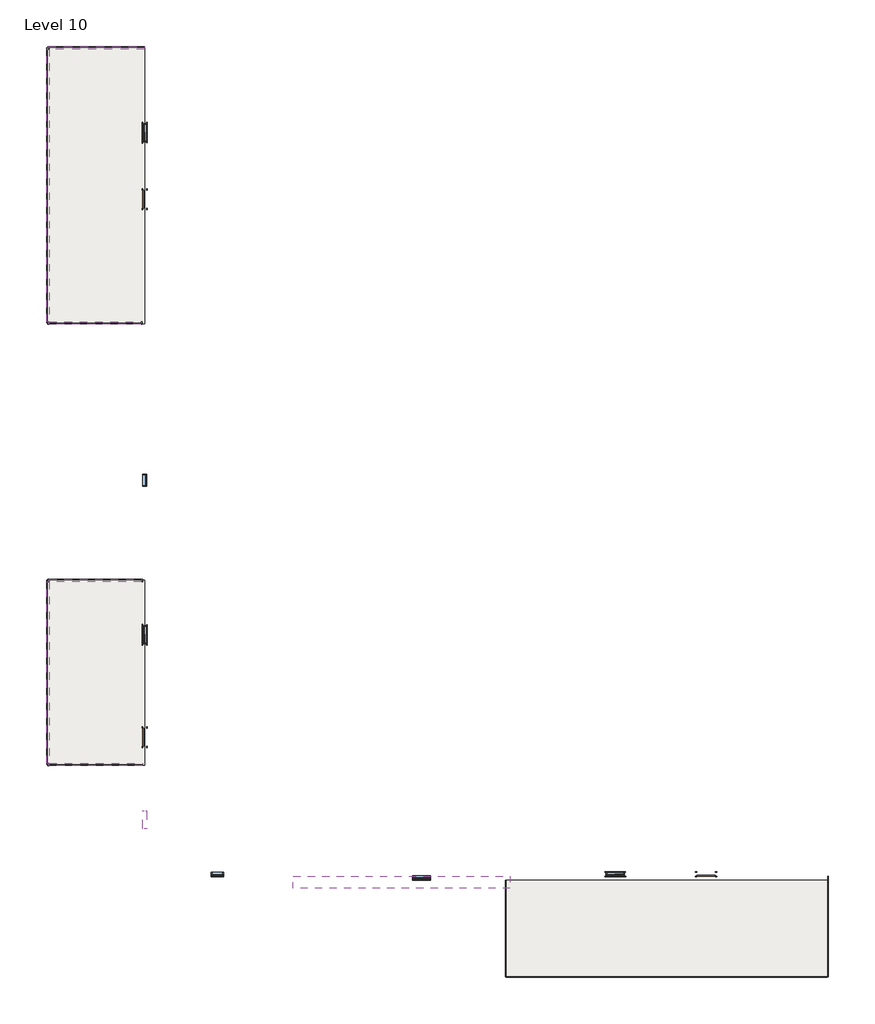
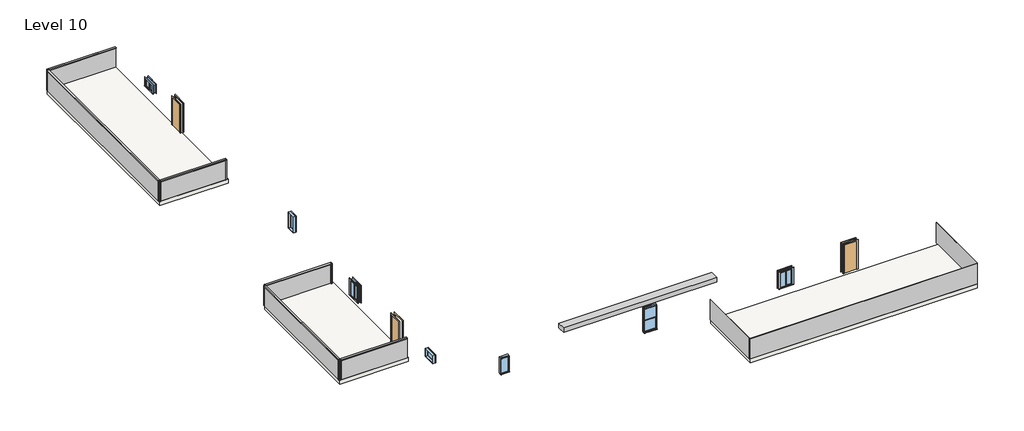
# One storey: 15 members, 9 plates, 7 windows, 3 doors, 3 slabs, 1 proxy.
"""IFC4 building model written with IfcOpenShell, lengths in millimetres."""

from ifc_helpers import new_model, si_unit, frame, origin, place, context, project, spatial, polyline, outline, extrude, transform, mapped, element, save
from components import generic_models_6_generic_models_6_4e89bfb7, door_54dd4da4, door_719f80de, member_4491d118, member_6d14b308, member_5c8c9790, member_b978f1c8, member_fc9bce7c, member_e4af79e9, member_f5ad0230, system_panel_glazed_dbf8c7ac, system_panel_glazed_4eae45b3, system_panel_glazed_9244b5db, system_panel_glazed_1f759628, system_panel_glazed_f6bd2989, system_panel_glazed_6e908680, system_panel_glazed_242742f8, system_panel_glazed_7dd8e57f, system_panel_glazed_8414a7a5, window_f274a882, window_80bd9af0, window_57c3ee1c, window_78885257, window_a4355bb3, window_54100e87

model = new_model("IFC4")

# Units and contexts
model_context = context("Model", 3, world=origin())
ifc_project = project(units=[si_unit("LENGTHUNIT", "METRE", prefix="MILLI")], contexts=[model_context])

# Site, building, storey
site = spatial("IfcSite", under=ifc_project)
building = spatial("IfcBuilding", under=site)
storey = spatial("IfcBuildingStorey", under=building, Name="Level 10", Elevation=16459.2)

# Proxy
placement = place(None, origin())
generic_models_6_generic_models_6_shape = generic_models_6_generic_models_6_4e89bfb7(model_context)
element("IfcBuildingElementProxy", 1, Name="Generic Models 6 : Generic Models 6", ObjectType="Generic Models 6 : Generic Models 6", at=placement, inside=storey, context=model_context, shape_type="MappedRepresentation", body=[
    mapped(generic_models_6_generic_models_6_shape, transform((0.0, 0.0, 0.0), x_axis=(1.0, 0.0, 0.0), y_axis=(0.0, 1.0, 0.0), z_axis=(0.0, 0.0, 1.0))),
])

# Doors
door_shape = door_54dd4da4(model_context)
element("IfcDoor", 2, ObjectType="Single-Flush : 36\" x 84\"", at=placement, inside=storey, context=model_context, shape_type="MappedRepresentation", body=[
    mapped(door_shape, transform((-15175.038074, 13190.2014639, 16459.2), x_axis=(0.0, 1.0, 0.0), y_axis=(-1.0, 0.0, 0.0), z_axis=(0.0, 0.0, 1.0))),
])
element("IfcDoor", 3, ObjectType="Single-Flush : 36\" x 84\"", at=placement, inside=storey, context=model_context, shape_type="MappedRepresentation", body=[
    mapped(door_shape, transform((-15175.038074, -13852.5915889, 16459.2), x_axis=(0.0, 1.0, 0.0), y_axis=(-1.0, 0.0, 0.0), z_axis=(0.0, 0.0, 1.0))),
])
door_2_shape = door_719f80de(model_context)
element("IfcDoor", 4, ObjectType="Single-Flush : 36\" x 84\"", at=placement, inside=storey, context=model_context, shape_type="MappedRepresentation", body=[
    mapped(door_2_shape, transform((13069.761926, -20744.1985361, 16459.2), x_axis=(1.0, 0.0, 0.0), y_axis=(0.0, 1.0, 0.0), z_axis=(0.0, 0.0, 1.0))),
])

# Members
member_shape = member_4491d118(model_context)
element("IfcMember", 5, ObjectType="Rectangular Mullion : 2.5\" x 5\" rectangular", at=placement, inside=storey, context=model_context, shape_type="MappedRepresentation", body=[
    mapped(member_shape, transform((-20051.838074, 6979.9014639, 16459.2), x_axis=(-1.0, 0.0, 0.0), y_axis=(0.0, 1.0, 0.0), z_axis=(0.0, 0.0, -1.0))),
])
element("IfcMember", 6, ObjectType="Rectangular Mullion : 2.5\" x 5\" rectangular", at=placement, inside=storey, context=model_context, shape_type="MappedRepresentation", body=[
    mapped(member_shape, transform((-20051.838074, 20810.2014639, 16459.2), x_axis=(0.0, 1.0, 0.0), y_axis=(1.0, 0.0, 0.0), z_axis=(0.0, 0.0, -1.0))),
])
element("IfcMember", 7, ObjectType="Rectangular Mullion : 2.5\" x 5\" rectangular", at=placement, inside=storey, context=model_context, shape_type="MappedRepresentation", body=[
    mapped(member_shape, transform((-20051.838074, -15224.1915889, 16459.2), x_axis=(-1.0, 0.0, 0.0), y_axis=(0.0, 1.0, 0.0), z_axis=(0.0, 0.0, -1.0))),
])
element("IfcMember", 8, ObjectType="Rectangular Mullion : 2.5\" x 5\" rectangular", at=placement, inside=storey, context=model_context, shape_type="MappedRepresentation", body=[
    mapped(member_shape, transform((-15276.638074, -5966.8213044, 16459.2), x_axis=(1.0, 0.0, 0.0), y_axis=(0.0, -1.0, 0.0), z_axis=(0.0, 0.0, -1.0))),
])
element("IfcMember", 9, ObjectType="Rectangular Mullion : 2.5\" x 5\" rectangular", at=placement, inside=storey, context=model_context, shape_type="MappedRepresentation", body=[
    mapped(member_shape, transform((-20051.838074, -5966.8213044, 16459.2), x_axis=(0.0, 1.0, 0.0), y_axis=(1.0, 0.0, 0.0), z_axis=(0.0, 0.0, -1.0))),
])
element("IfcMember", 10, ObjectType="Rectangular Mullion : 2.5\" x 5\" rectangular", at=placement, inside=storey, context=model_context, shape_type="MappedRepresentation", body=[
    mapped(member_shape, transform((-20051.838074, 6979.9014639, 17983.2), x_axis=(0.0, -1.0, 0.0), y_axis=(1.0, 0.0, 0.0), z_axis=(0.0, 0.0, 1.0))),
])
element("IfcMember", 11, ObjectType="Rectangular Mullion : 2.5\" x 5\" rectangular", at=placement, inside=storey, context=model_context, shape_type="MappedRepresentation", body=[
    mapped(member_shape, transform((-15295.688074, 6979.9014639, 17983.2), x_axis=(1.0, 0.0, 0.0), y_axis=(0.0, 1.0, 0.0), z_axis=(0.0, 0.0, 1.0))),
])
element("IfcMember", 12, ObjectType="Rectangular Mullion : 2.5\" x 5\" rectangular", at=placement, inside=storey, context=model_context, shape_type="MappedRepresentation", body=[
    mapped(member_shape, transform((-20051.838074, -15224.1915889, 17983.2), x_axis=(0.0, -1.0, 0.0), y_axis=(1.0, 0.0, 0.0), z_axis=(0.0, 0.0, 1.0))),
])
element("IfcMember", 13, ObjectType="Rectangular Mullion : 2.5\" x 5\" rectangular", at=placement, inside=storey, context=model_context, shape_type="MappedRepresentation", body=[
    mapped(member_shape, transform((-20051.838074, -5966.8213044, 17983.2), x_axis=(-1.0, 0.0, 0.0), y_axis=(0.0, -1.0, 0.0), z_axis=(0.0, 0.0, 1.0))),
])
member_2_shape = member_6d14b308(model_context)
element("IfcMember", 14, ObjectType="Rectangular Mullion : 2.5\" x 5\" rectangular", at=placement, inside=storey, context=model_context, shape_type="MappedRepresentation", body=[
    mapped(member_2_shape, transform((-15340.138074, -5966.8213044, 17983.2), x_axis=(0.0, 0.0, 1.0), y_axis=(0.0, -1.0, 0.0), z_axis=(1.0, 0.0, 0.0))),
])
member_3_shape = member_5c8c9790(model_context)
element("IfcMember", 15, ObjectType="Rectangular Mullion : 2.5\" x 5\" rectangular", at=placement, inside=storey, context=model_context, shape_type="MappedRepresentation", body=[
    mapped(member_3_shape, transform((-19988.338074, 6979.9014639, 17983.2), x_axis=(0.0, 0.0, 1.0), y_axis=(0.0, 1.0, 0.0), z_axis=(-1.0, 0.0, 0.0))),
])
member_4_shape = member_b978f1c8(model_context)
element("IfcMember", 16, ObjectType="Rectangular Mullion : 2.5\" x 5\" rectangular", at=placement, inside=storey, context=model_context, shape_type="MappedRepresentation", body=[
    mapped(member_4_shape, transform((-20051.838074, 20746.7014639, 17983.2), x_axis=(0.0, 0.0, 1.0), y_axis=(1.0, 0.0, 0.0), z_axis=(0.0, 1.0, 0.0))),
])
member_5_shape = member_fc9bce7c(model_context)
element("IfcMember", 17, ObjectType="Rectangular Mullion : 2.5\" x 5\" rectangular", at=placement, inside=storey, context=model_context, shape_type="MappedRepresentation", body=[
    mapped(member_5_shape, transform((-15175.038074, 20810.2014639, 17983.2), x_axis=(0.0, 0.0, 1.0), y_axis=(0.0, -1.0, 0.0), z_axis=(1.0, 0.0, 0.0))),
])
member_6_shape = member_e4af79e9(model_context)
element("IfcMember", 18, ObjectType="Rectangular Mullion : 2.5\" x 5\" rectangular", at=placement, inside=storey, context=model_context, shape_type="MappedRepresentation", body=[
    mapped(member_6_shape, transform((-19988.338074, -15224.1915889, 17983.2), x_axis=(0.0, 0.0, 1.0), y_axis=(0.0, 1.0, 0.0), z_axis=(-1.0, 0.0, 0.0))),
])
member_7_shape = member_f5ad0230(model_context)
element("IfcMember", 19, ObjectType="Rectangular Mullion : 2.5\" x 5\" rectangular", at=placement, inside=storey, context=model_context, shape_type="MappedRepresentation", body=[
    mapped(member_7_shape, transform((-20051.838074, -6030.3213044, 17983.2), x_axis=(0.0, 0.0, 1.0), y_axis=(1.0, 0.0, 0.0), z_axis=(0.0, 1.0, 0.0))),
])

# Plates
system_panel_glazed_shape = system_panel_glazed_dbf8c7ac(model_context)
element("IfcPlate", 20, ObjectType="System Panel : Glazed", at=placement, inside=storey, context=model_context, shape_type="MappedRepresentation", body=[
    mapped(system_panel_glazed_shape, transform((11088.561926, -25891.2590157, 16459.2), x_axis=(-1.0, 0.0, 0.0), y_axis=(0.0, -1.0, 0.0), z_axis=(0.0, 0.0, 1.0))),
])
system_panel_glazed_2_shape = system_panel_glazed_4eae45b3(model_context)
element("IfcPlate", 21, ObjectType="System Panel : Glazed", at=placement, inside=storey, context=model_context, shape_type="MappedRepresentation", body=[
    mapped(system_panel_glazed_2_shape, transform((3011.361926, -23470.1287759, 16459.2), x_axis=(0.0, 1.0, 0.0), y_axis=(-1.0, 0.0, 0.0), z_axis=(0.0, 0.0, 1.0))),
])
system_panel_glazed_3_shape = system_panel_glazed_9244b5db(model_context)
element("IfcPlate", 22, ObjectType="System Panel : Glazed", at=placement, inside=storey, context=model_context, shape_type="MappedRepresentation", body=[
    mapped(system_panel_glazed_3_shape, transform((19165.761926, -23368.5287759, 16459.2), x_axis=(0.0, -1.0, 0.0), y_axis=(1.0, 0.0, 0.0), z_axis=(0.0, 0.0, 1.0))),
])
system_panel_glazed_4_shape = system_panel_glazed_1f759628(model_context)
element("IfcPlate", 23, ObjectType="System Panel : Glazed", at=placement, inside=storey, context=model_context, shape_type="MappedRepresentation", body=[
    mapped(system_panel_glazed_4_shape, transform((-17664.238074, -5966.8213044, 16459.2), x_axis=(1.0, 0.0, 0.0), y_axis=(0.0, 1.0, 0.0), z_axis=(0.0, 0.0, 1.0))),
])
system_panel_glazed_5_shape = system_panel_glazed_f6bd2989(model_context)
element("IfcPlate", 24, ObjectType="System Panel : Glazed", at=placement, inside=storey, context=model_context, shape_type="MappedRepresentation", body=[
    mapped(system_panel_glazed_5_shape, transform((-17673.763074, 6979.9014639, 16459.2), x_axis=(-1.0, 0.0, 0.0), y_axis=(0.0, -1.0, 0.0), z_axis=(0.0, 0.0, 1.0))),
])
system_panel_glazed_6_shape = system_panel_glazed_6e908680(model_context)
element("IfcPlate", 25, ObjectType="System Panel : Glazed", at=placement, inside=storey, context=model_context, shape_type="MappedRepresentation", body=[
    mapped(system_panel_glazed_6_shape, transform((-20051.838074, 13895.0514639, 16459.2), x_axis=(0.0, 1.0, 0.0), y_axis=(-1.0, 0.0, 0.0), z_axis=(0.0, 0.0, 1.0))),
])
system_panel_glazed_7_shape = system_panel_glazed_242742f8(model_context)
element("IfcPlate", 26, ObjectType="System Panel : Glazed", at=placement, inside=storey, context=model_context, shape_type="MappedRepresentation", body=[
    mapped(system_panel_glazed_7_shape, transform((-17613.438074, 20810.2014639, 16459.2), x_axis=(1.0, 0.0, 0.0), y_axis=(0.0, 1.0, 0.0), z_axis=(0.0, 0.0, 1.0))),
])
system_panel_glazed_8_shape = system_panel_glazed_7dd8e57f(model_context)
element("IfcPlate", 27, ObjectType="System Panel : Glazed", at=placement, inside=storey, context=model_context, shape_type="MappedRepresentation", body=[
    mapped(system_panel_glazed_8_shape, transform((-17632.488074, -15224.1915889, 16459.2), x_axis=(-1.0, 0.0, 0.0), y_axis=(0.0, -1.0, 0.0), z_axis=(0.0, 0.0, 1.0))),
])
system_panel_glazed_9_shape = system_panel_glazed_8414a7a5(model_context)
element("IfcPlate", 28, ObjectType="System Panel : Glazed", at=placement, inside=storey, context=model_context, shape_type="MappedRepresentation", body=[
    mapped(system_panel_glazed_9_shape, transform((-20051.838074, -10595.5064466, 16459.2), x_axis=(0.0, 1.0, 0.0), y_axis=(-1.0, 0.0, 0.0), z_axis=(0.0, 0.0, 1.0))),
])

# Slabs
element("IfcSlab", 29, ObjectType="Generic - 12\"", at=placement, inside=storey, context=model_context, shape_type="SweptSolid", body=[
    extrude(outline(polyline([(3011.361926, -21048.9985361), (19165.761926, -21048.9985361), (19165.761926, -25925.7985361), (3011.361926, -25925.7985361), (3011.361926, -21048.9985361)])), frame((0.0, 0.0, 16154.4), z_axis=(0.0, 0.0, 1.0), x_axis=(1.0, 0.0, 0.0)), (0.0, 0.0, 1.0), 304.8),
])
element("IfcSlab", 30, ObjectType="Generic - 12\"", at=placement, inside=storey, context=model_context, shape_type="SweptSolid", body=[
    extrude(outline(polyline([(-20051.838074, -15263.2213044), (-20051.838074, -5966.8213044), (-15175.038074, -5966.8213044), (-15175.038074, -15263.2213044), (-20051.838074, -15263.2213044)])), frame((0.0, 0.0, 16154.4), z_axis=(0.0, 0.0, 1.0), x_axis=(1.0, 0.0, 0.0)), (0.0, 0.0, 1.0), 304.8),
])
element("IfcSlab", 31, ObjectType="Generic - 12\"", at=placement, inside=storey, context=model_context, shape_type="SweptSolid", body=[
    extrude(outline(polyline([(-20051.838074, 20810.2014639), (-15175.038074, 20810.2014639), (-15175.038074, 6941.8014639), (-20051.838074, 6941.8014639), (-20051.838074, 20810.2014639)])), frame((0.0, 0.0, 16154.4), z_axis=(0.0, 0.0, 1.0), x_axis=(1.0, 0.0, 0.0)), (0.0, 0.0, 1.0), 304.8),
])

# Windows
window_shape = window_f274a882(model_context)
element("IfcWindow", 32, ObjectType="Double Hung : 36\" x 72\"", at=placement, inside=storey, context=model_context, shape_type="MappedRepresentation", body=[
    mapped(window_shape, transform((-1255.838074, -20921.9985361, 16763.7012618), x_axis=(-1.0, 0.0, 0.0), y_axis=(0.0, -1.0, 0.0), z_axis=(0.0, 0.0, 1.0))),
])
window_2_shape = window_80bd9af0(model_context)
element("IfcWindow", 33, ObjectType="Fixed : 24\" x 48\"", at=placement, inside=storey, context=model_context, shape_type="MappedRepresentation", body=[
    mapped(window_2_shape, transform((-15175.038074, -975.7213044, 16459.2), x_axis=(0.0, -1.0, 0.0), y_axis=(1.0, 0.0, 0.0), z_axis=(0.0, 0.0, 1.0))),
])
window_3_shape = window_57c3ee1c(model_context)
element("IfcWindow", 34, ObjectType="Fixed : 36\" x 24\"", at=placement, inside=storey, context=model_context, shape_type="MappedRepresentation", body=[
    mapped(window_3_shape, transform((-15175.038074, -18041.8099202, 17047.6304295), x_axis=(0.0, -1.0, 0.0), y_axis=(1.0, 0.0, 0.0), z_axis=(0.0, 0.0, 1.0))),
])
window_4_shape = window_78885257(model_context)
element("IfcWindow", 35, ObjectType="Instance - Fixed : 24\" x 48\"", at=placement, inside=storey, context=model_context, shape_type="MappedRepresentation", body=[
    mapped(window_4_shape, transform((-11555.538074, -20744.1985361, 16459.2), x_axis=(-1.0, 0.0, 0.0), y_axis=(0.0, -1.0, 0.0), z_axis=(0.0, 0.0, 1.0))),
])
window_5_shape = window_a4355bb3(model_context)
element("IfcWindow", 36, ObjectType="Slider with Trim : 36\" x 24\"", at=placement, inside=storey, context=model_context, shape_type="MappedRepresentation", body=[
    mapped(window_5_shape, transform((-15175.038074, 16543.0014639, 16459.2), x_axis=(0.0, 1.0, 0.0), y_axis=(-1.0, 0.0, 0.0), z_axis=(0.0, 0.0, 1.0))),
])
window_6_shape = window_54100e87(model_context)
element("IfcWindow", 37, ObjectType="Slider with Trim : 36\" x 48\"", at=placement, inside=storey, context=model_context, shape_type="MappedRepresentation", body=[
    mapped(window_6_shape, transform((8497.761926, -20744.1985361, 15972.7578988), x_axis=(-1.0, 0.0, 0.0), y_axis=(0.0, -1.0, 0.0), z_axis=(0.0, 0.0, 1.0))),
])
element("IfcWindow", 38, ObjectType="Slider with Trim : 36\" x 48\"", at=placement, inside=storey, context=model_context, shape_type="MappedRepresentation", body=[
    mapped(window_6_shape, transform((-15175.038074, -8710.0213044, 16003.7013379), x_axis=(0.0, 1.0, 0.0), y_axis=(-1.0, 0.0, 0.0), z_axis=(0.0, 0.0, 1.0))),
])

save(model, "model.ifc")

# Revit data of these elements
# Type "Single-Flush : 36\" x 84\""
#   Type Mark = "1"
#   Construction Type Id = "MDOOR"
#   Assembly Code = "C1020"
#   Analytic Construction = "Metal"
#   Thickness = 0' - 2"
#   Heat Transfer Coefficient (U) = 0.651978 BTU/(h·ft²·°F)
#   Height = 7' - 0"
#   Trim Projection Ext = 0' - 1"
#   Trim Projection Int = 0' - 1"
#   Trim Width = 0' - 3"
#   Width = 3' - 0"
#   Define Thermal Properties by = 1
#   Door Material = Door - Panel
#   Frame Material = Door - Frame
#   Visual Light Transmittance = 0
#   Solar Heat Gain Coefficient = 0
#   Function = (empty or 0)
#   Wall Closure = (empty or 0)
# Type "Rectangular Mullion : 2.5\" x 5\" rectangular"
#   built-in parameter 1007304 = 0.416667 (stored number, unit not read)
#   built-in parameter 1007301 = 0.104167 (stored number, unit not read)
#   built-in parameter 1007300 = 0.104167 (stored number, unit not read)
# Type "System Panel : Glazed"
#   Construction Type Id = "GSP4R"
#   Analytic Construction = "1/8 in Pilkington single glazing"
#   Visual Light Transmittance = 0.9
#   Solar Heat Gain Coefficient = 0.86
#   Heat Transfer Coefficient (U) = 1.18115 BTU/(h·ft²·°F)
# Type "Generic - 12\""
#   Assembly Code = "B1010"
#   Function = 0
#   Layers, outside or top first: 1' - 0" no material (function 1)
# Type "Double Hung : 36\" x 72\""
#   Type Mark = "18"
#   Construction Type Id = "GSP4R"
#   Assembly Code = "B2020100"
#   Analytic Construction = "1/8 in Pilkington single glazing"
#   Visual Light Transmittance = 0.9
#   Solar Heat Gain Coefficient = 0.78
#   Heat Transfer Coefficient (U) = 0.6496 BTU/(h·ft²·°F)
#   Height = 6' - 0"
#   Default Sill Height = 1' - 0"
#   Width = 3' - 0"
#   Window Inset = 0' - 0 3/4"
#   Define Thermal Properties by = 1
#   Glass Pane Material = Glass
#   Sash Material = Sash
#   Description = (empty or 0)
#   Wall Closure = (empty or 0)
# Type "Fixed : 24\" x 48\""
#   Type Mark = "2"
#   Construction Type Id = "GSP4R"
#   Assembly Code = "B2020100"
#   Analytic Construction = "1/8 in Pilkington single glazing"
#   Visual Light Transmittance = 0.9
#   Solar Heat Gain Coefficient = 0.78
#   Heat Transfer Coefficient (U) = 0.6496 BTU/(h·ft²·°F)
#   Height = 4' - 0"
#   Default Sill Height = 3' - 0"
#   Width = 2' - 0"
#   Window Inset = 0' - 0 3/4"
#   Define Thermal Properties by = 1
#   Glass Pane Material = Glass
#   Sash Material = Sash
#   Wall Closure = (empty or 0)
# Type "Fixed : 36\" x 24\""
#   Type Mark = "8"
#   Construction Type Id = "GSP4R"
#   Assembly Code = "B2020100"
#   Analytic Construction = "1/8 in Pilkington single glazing"
#   Visual Light Transmittance = 0.9
#   Solar Heat Gain Coefficient = 0.78
#   Heat Transfer Coefficient (U) = 0.6496 BTU/(h·ft²·°F)
#   Height = 2' - 0"
#   Default Sill Height = 3' - 0"
#   Width = 3' - 0"
#   Window Inset = 0' - 0 3/4"
#   Define Thermal Properties by = 1
#   Glass Pane Material = Glass
#   Sash Material = Sash
#   Wall Closure = (empty or 0)
# Type "Instance - Fixed : 24\" x 48\""
#   Type Mark = "19"
#   Construction Type Id = "GSP4R"
#   Assembly Code = "B2020100"
#   Analytic Construction = "1/8 in Pilkington single glazing"
#   Visual Light Transmittance = 0.9
#   Thermal Resistance (R) = 0.8466 (h·ft²·°F)/BTU
#   Solar Heat Gain Coefficient = 0.86
#   Heat Transfer Coefficient (U) = 1.1812 BTU/(h·ft²·°F)
#   Height [instance default] = 4' - 0"
#   Default Sill Height = 3' - 0"
#   Width [instance default] = 2' - 0"
#   Window Inset = 0' - 0 3/4"
#   Define Thermal Properties by = 1
#   Glass Pane Material = Glass
#   Sash Material = Sash
#   Wall Closure = (empty or 0)
# Type "Slider with Trim : 36\" x 24\""
#   Type Mark = "23"
#   Construction Type Id = "GSP4R"
#   Assembly Code = "B2020100"
#   Analytic Construction = "1/8 in Pilkington single glazing"
#   Visual Light Transmittance = 0.9
#   Solar Heat Gain Coefficient = 0.78
#   Heat Transfer Coefficient (U) = 0.6496 BTU/(h·ft²·°F)
#   Height = 2' - 0"
#   Default Sill Height = 3' - 0"
#   Trim Projection - Ext. = 0' - 0 3/4"
#   Trim Projection - Int. = 0' - 0 3/4"
#   Trim Width - Exterior = 0' - 3 1/2"
#   Trim Width - Interior = 0' - 3 1/2"
#   Width = 3' - 0"
#   Window Inset = 0' - 0 3/4"
#   Define Thermal Properties by = 1
#   Glass Pane Material = Glass
#   Sash Material = Sash
#   Trim Exterior Material = Trim
#   Trim Interior Material = Trim
#   Wall Closure = (empty or 0)
# Type "Slider with Trim : 36\" x 48\""
#   Type Mark = "22"
#   Construction Type Id = "GSP4R"
#   Assembly Code = "B2020100"
#   Analytic Construction = "1/8 in Pilkington single glazing"
#   Visual Light Transmittance = 0.9
#   Solar Heat Gain Coefficient = 0.78
#   Heat Transfer Coefficient (U) = 0.6496 BTU/(h·ft²·°F)
#   Height = 4' - 0"
#   Default Sill Height = 3' - 0"
#   Trim Projection - Ext. = 0' - 0 3/4"
#   Trim Projection - Int. = 0' - 0 3/4"
#   Trim Width - Exterior = 0' - 3 1/2"
#   Trim Width - Interior = 0' - 3 1/2"
#   Width = 3' - 0"
#   Window Inset = 0' - 0 3/4"
#   Define Thermal Properties by = 1
#   Glass Pane Material = Glass
#   Sash Material = Sash
#   Trim Exterior Material = Trim
#   Trim Interior Material = Trim
#   Wall Closure = (empty or 0)
# Element 1 (IfcBuildingElementProxy, "Generic Models 6 : Generic Models 6")
#   Phase Created = New Construction
# Elements 2, 3, 4 (IfcDoor, "Single-Flush : 36\" x 84\"")
#   Phase Created = New Construction
#   Materials on its faces: "Door - Frame", "Door - Panel"
# Elements 5, 6, 7, 8, 9, 10, 11, 12, 13, 14, 15, 16, 17, 18, 19 (IfcMember, "Rectangular Mullion : 2.5\" x 5\" rectangular")
#   Phase Created = New Construction
#   Materials on its faces: "Aluminum"
# Elements 20, 21, 22, 23, 24, 25, 26, 27, 28 (IfcPlate, "System Panel : Glazed")
#   Phase Created = New Construction
#   Materials on its faces: "Glass"
# Elements 29, 30, 31 (IfcSlab, "Generic - 12\"")
#   built-in parameter 1001955 = 3.14159 (stored number, unit not read)
#   Height Offset From Level = 0' - 0"
#   Phase Created = New Construction
#   Materials on its faces: "Default Floor"
# Element 32 (IfcWindow, "Double Hung : 36\" x 72\"")
#   Mark = "7"
#   Phase Created = New Construction
#   Materials on its faces: "Sash", "Glass"
# Element 33 (IfcWindow, "Fixed : 24\" x 48\"")
#   Mark = "51"
#   Phase Created = New Construction
#   Materials on its faces: "Sash", "Glass"
# Element 34 (IfcWindow, "Fixed : 36\" x 24\"")
#   Mark = "73"
#   Phase Created = New Construction
#   Materials on its faces: "Sash", "Glass"
# Element 35 (IfcWindow, "Instance - Fixed : 24\" x 48\"")
#   Mark = "18"
#   Width = 2' - 0"
#   Height = 4' - 0"
#   Phase Created = New Construction
#   Materials on its faces: "Sash", "Glass"
# Element 36 (IfcWindow, "Slider with Trim : 36\" x 24\"")
#   Mark = "62"
#   Phase Created = New Construction
#   Materials on its faces: "Sash", "Trim", "Glass"
# Element 37 (IfcWindow, "Slider with Trim : 36\" x 48\"")
#   Mark = "29"
#   Phase Created = New Construction
#   Materials on its faces: "Sash", "Trim", "Glass"
# Element 38 (IfcWindow, "Slider with Trim : 36\" x 48\"")
#   Mark = "40"
#   Phase Created = New Construction
#   Materials on its faces: "Sash", "Trim", "Glass"
# Materials
#   "Door - Panel": class "Wood", colour RGB 210 159 95, transparency 0
#   "Door - Frame": colour RGB 118 70 51, transparency 0
#   "Glass": class "Glass", colour RGB 0 128 192, transparency 0.75, Description = "Soda Lime Glass", Cost = 0
#   "Sash": class "Wood", colour RGB 224 178 126, transparency 0
#   "Trim": class "Wood", colour RGB 224 178 126, transparency 0
#   "Aluminum": class "Metal", colour RGB 247 247 247, transparency 0, Description = "Aluminum 6061", Cost = 0
#   "Default Floor": colour RGB 128 128 128, transparency 0
